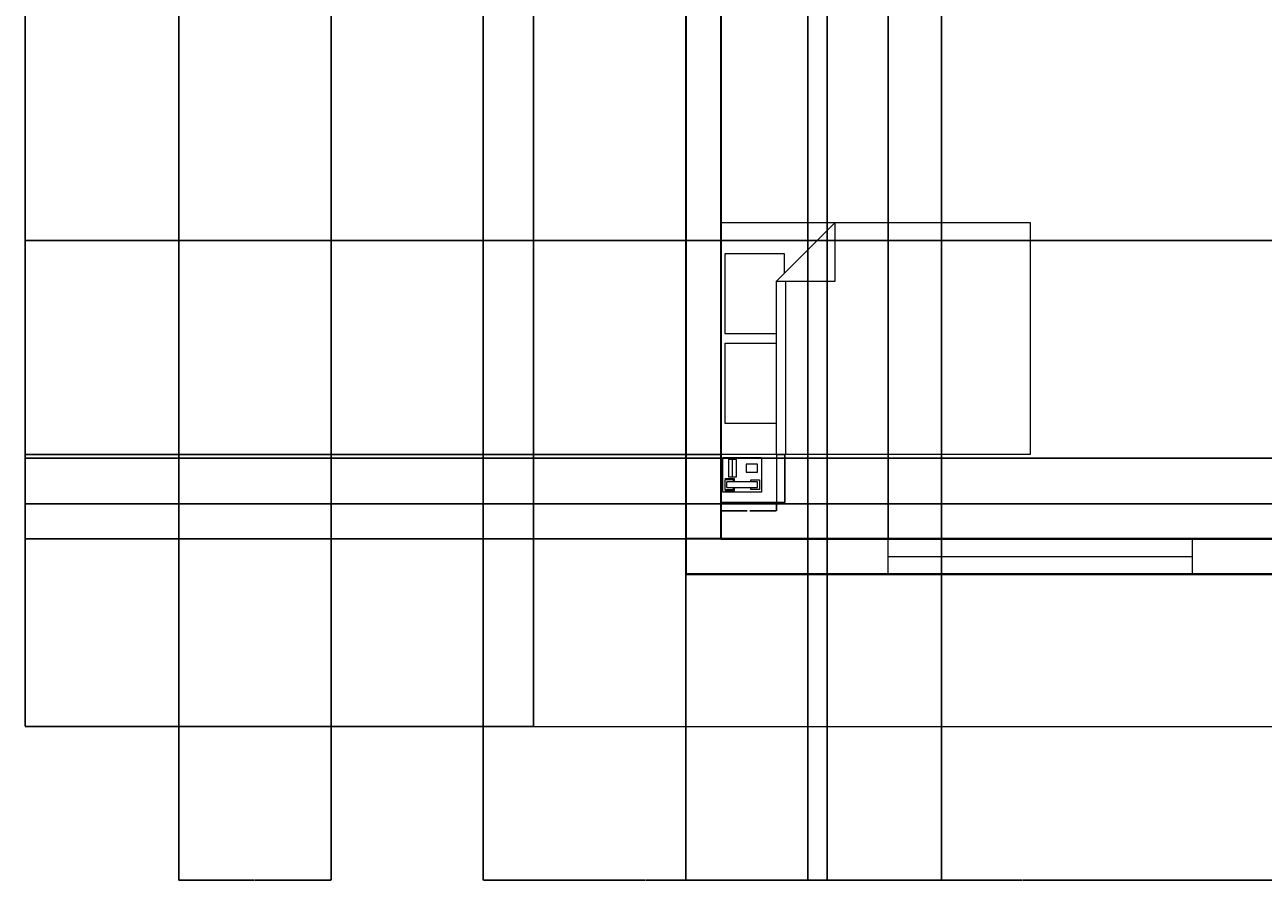
# Model space of a CAD drawing. Units: millimetres. Extents: x -8052 to 19968, y -37825 to -17505.
# Tile 1 of 10: x -8052 to 84, y -37825 to -32209. Entities that reach past the tile are written whole.
import ezdxf

# ---------------------------------------------------------------- set-up
doc = ezdxf.new("R2010")
doc.units = ezdxf.units.MM
doc.header["$MEASUREMENT"] = 0
for name, color, linetype, lineweight in [('A-ANNO-DIMS', 2, 'Continuous', 18), ('A-EQPM', 8, 'Continuous', 18), ('A-FLOR', 8, 'Continuous', 18), ('A-FURN', 8, 'Continuous', 18), ('A-GLAZ', 4, 'Continuous', 18), ('A-WALL', 7, 'Continuous', 35)]:
    doc.layers.add(name, color=color, linetype=linetype, lineweight=lineweight)
doc.styles.get("Standard").update_dxf_attribs({"font": 'arial.ttf'})
doc.dimstyles.get("Standard").update_dxf_attribs({"dimtxt": 1.054, "dimasz": 1.055, "dimexe": 0.18, "dimexo": 0.0625, "dimgap": 0.09, "dimtad": 0, "dimtih": 1, "dimtoh": 1, "dimdec": 4, "dimzin": 0, "dimdsep": 46, "dimtxsty": 'Standard', "dimcen": 0.09, "dimadec": 0, "dimazin": 0, "dimtfac": 1, "dimtdec": 4, "dimtofl": 0, "dimtmove": 0, "dimatfit": 3, "dimfxl": 1, "dimtolj": 1, "dimtzin": 0, "dimarcsym": 0})

# ---------------------------------------------------------------- blocks, each defined once
blk = doc.blocks.new('Bed - Queen')
for p, q in [((0, -80.00003), (0, 0)), ((0, 0), (59.99999, 0)), ((59.99999, 0), (59.99999, -80.00003)), ((7.99999, -1.2), (28.79998, -1.2)), ((7.99999, -14.4), (7.99999, -1.2)), ((28.79998, -1.2), (28.79998, -14.4)), ((31.19999, -1.2), (51.99999, -1.2)), ((31.19999, -14.4), (31.19999, -1.2)), ((51.99999, -1.2), (51.99999, -16.4)), ((0, -14.4), (44.8, -14.4)), ((59.99999, -29.6), (44.8, -14.4)), ((44.8, -14.4), (44.8, -29.6)), ((44.8, -16.8), (0, -16.8)), ((51.99999, -16.4), (46.79936, -16.4)), ((44.8, -29.6), (59.99999, -29.6)), ((59.99999, -80.00003), (0, -80.00003))]:
    blk.add_line(p, q)
blk = doc.blocks.new('Phone - Desk')
for p, q in [((-4.5, -5), (-4.5, 5)), ((-4.5, 5), (4.5, 5)), ((-4, 4.5), (-4, 2)), ((-3.75, 4.5), (-3.75, 2.25)), ((-1.25, 4.5), (-3.75, 4.5)), ((-3.25, 4), (-3.25, -4)), ((-3.25, 4), (-1.75, 4)), ((-1.75, -4), (-1.75, 4)), ((-1.25, 2.25), (-1.25, 4.5)), ((-1, 2), (-1, 4.5)), ((4, 3.5), (-0.5, 3.5)), ((-0.5, 3.5), (-0.5, 1.5)), ((4, 1.5), (4, 3.5)), ((4.5, 5), (4.5, -5)), ((-4, 2), (-3.25, 2)), ((-3.75, 2.25), (-3.25, 2.25)), ((-1.75, 2.25), (-1.25, 2.25)), ((-1.75, 2), (-1, 2)), ((-0.5, 2.5), (4, 2.5)), ((-0.5, 1.5), (4, 1.5)), ((-3.75, -2.25), (-3.25, -2.25)), ((-3.75, -4.5), (-3.75, -2.25)), ((-1.75, -2.25), (-1.25, -2.25)), ((-1.25, -2.25), (-1.25, -4.5)), ((2.75, -1), (0.75, -1)), ((0.75, -1), (0.75, -4)), ((2.75, -4), (2.75, -1)), ((4.5, -5), (-4.5, -5)), ((-1.25, -4.5), (-3.75, -4.5)), ((-3.25, -4), (-1.75, -4)), ((0.75, -4), (2.75, -4))]:
    blk.add_line(p, q)
blk = doc.blocks.new('TABLE-BEDSIDE')
for p, q in [((365.8, 315.3), (365.8, 0)), ((365.8, 0), (0, 0))]:
    blk.add_line(p, q)
blk = doc.blocks.new('WIN-2000')
for p, q in [((0, 0), (0, 230)), ((2000, 0), (2000, 230)), ((0, 115), (2000, 115))]:
    blk.add_line(p, q)
blk = doc.blocks.new('*D50')
at = {"layer": 'A-ANNO-DIMS', "color": 0, "lineweight": -2, "transparency": 16777216}
for p, q in [((-3480, -35345.8), (-3480, -35400.8)), ((-3114.3, -35345.8), (-3114.3, -35400.8)), ((-3479, -35400.6), (-3306.2, -35400.6)), ((-3115.3, -35400.6), (-3288.1, -35400.6))]:
    blk.add_line(p, q, dxfattribs=at)
at = {"layer": 'A-ANNO-DIMS', "color": 0, "lineweight": 100, "transparency": 16777216}
for points in [[(-3479, -35400.5), (-3479, -35400.8), (-3480, -35400.6)], [(-3115.3, -35400.5), (-3115.3, -35400.8), (-3114.3, -35400.6)]]:
    blk.add_solid(points, dxfattribs=at)
at = {"layer": 'Defpoints', "color": 0, "lineweight": 100, "transparency": 16777216}
for p in [(-3480, -35345.8), (-3114.3, -35345.8), (-3114.3, -35400.6)]:
    blk.add_point(p, dxfattribs=at)
at = {"layer": 'A-ANNO-DIMS', "color": 0, "transparency": 16777216, "insert": (-3297.1, -35400.6), "char_height": 1.054, "attachment_point": 5}
blk.add_mtext('\\A1;BEDSIDE TABLE 366 TYP.', dxfattribs=at)
blk = doc.blocks.new('*D51')
at = {"layer": 'A-ANNO-DIMS', "color": 0, "lineweight": -2, "transparency": 16777216}
for p, q in [((-3114.2, -35030.5), (-3059.2, -35030.5)), ((-3059.4, -35031.6), (-3059.4, -35187.5)), ((-3059.4, -35344.7), (-3059.4, -35188.8)), ((-3114.2, -35345.8), (-3059.2, -35345.8))]:
    blk.add_line(p, q, dxfattribs=at)
at = {"layer": 'A-ANNO-DIMS', "color": 0, "lineweight": 100, "transparency": 16777216}
for points in [[(-3059.6, -35031.6), (-3059.2, -35031.6), (-3059.4, -35030.5)], [(-3059.6, -35344.7), (-3059.2, -35344.7), (-3059.4, -35345.8)]]:
    blk.add_solid(points, dxfattribs=at)
at = {"layer": 'Defpoints', "color": 0, "lineweight": 100, "transparency": 16777216}
for p in [(-3114.3, -35030.5), (-3059.4, -35030.5), (-3114.3, -35345.8)]:
    blk.add_point(p, dxfattribs=at)
at = {"layer": 'A-ANNO-DIMS', "color": 0, "transparency": 16777216, "insert": (-3059.4, -35188.1), "char_height": 1.054, "attachment_point": 5}
blk.add_mtext('\\A1;315 TYP.', dxfattribs=at)
blk = doc.blocks.new('*D85')
at = {"layer": 'A-ANNO-DIMS', "color": 0, "lineweight": -2, "transparency": 16777216}
for p, q in [((-7040.1, -18514.8), (-8049.7, -18514.8)), ((-8049.5, -18515.9), (-8049.5, -27664.2)), ((-8049.5, -36813.8), (-8049.5, -27665.5)), ((-4710.1, -36814.8), (-8049.7, -36814.8))]:
    blk.add_line(p, q, dxfattribs=at)
at = {"layer": 'A-ANNO-DIMS', "color": 0, "lineweight": 100, "transparency": 16777216}
for points in [[(-8049.7, -18515.9), (-8049.3, -18515.9), (-8049.5, -18514.8)], [(-8049.7, -36813.8), (-8049.3, -36813.8), (-8049.5, -36814.8)]]:
    blk.add_solid(points, dxfattribs=at)
at = {"layer": 'Defpoints', "color": 0, "lineweight": 100, "transparency": 16777216}
for p in [(-7040, -18514.8), (-8049.5, -36814.8), (-4710, -36814.8)]:
    blk.add_point(p, dxfattribs=at)
at = {"layer": 'A-ANNO-DIMS', "color": 0, "transparency": 16777216, "insert": (-8049.5, -27664.8), "char_height": 1.05, "attachment_point": 5}
blk.add_mtext('\\A1;18300', dxfattribs=at)
blk = doc.blocks.new('*D86')
at = {"layer": 'A-ANNO-DIMS', "color": 0, "lineweight": -2, "transparency": 16777216}
for p, q in [((-7040, -18514.9), (-7040, -37824.5)), ((-6040, -19514.9), (-6040, -37824.5)), ((-7039, -37824.3), (-6541.6, -37824.3)), ((-6041.1, -37824.3), (-6538.4, -37824.3))]:
    blk.add_line(p, q, dxfattribs=at)
at = {"layer": 'A-ANNO-DIMS', "color": 0, "lineweight": 100, "transparency": 16777216}
for points in [[(-7039, -37824.2), (-7039, -37824.5), (-7040, -37824.3)], [(-6041.1, -37824.2), (-6041.1, -37824.5), (-6040, -37824.3)]]:
    blk.add_solid(points, dxfattribs=at)
at = {"layer": 'Defpoints', "color": 0, "lineweight": 100, "transparency": 16777216}
for p in [(-7040, -18514.8), (-6040, -19514.8), (-6040, -37824.3)]:
    blk.add_point(p, dxfattribs=at)
at = {"layer": 'A-ANNO-DIMS', "color": 0, "transparency": 16777216, "insert": (-6540, -37824.3), "char_height": 1.05, "attachment_point": 5}
blk.add_mtext('\\A1;1000', dxfattribs=at)
blk = doc.blocks.new('*D94')
at = {"layer": 'A-ANNO-DIMS', "color": 0, "lineweight": -2, "transparency": 16777216}
for p, q in [((-2780, -20744.9), (-2780, -37824.5)), ((-2030, -20744.9), (-2030, -37824.5)), ((-2779, -37824.3), (-2406.3, -37824.3)), ((-2031.1, -37824.3), (-2403.8, -37824.3))]:
    blk.add_line(p, q, dxfattribs=at)
at = {"layer": 'A-ANNO-DIMS', "color": 0, "lineweight": 100, "transparency": 16777216}
for points in [[(-2779, -37824.2), (-2779, -37824.5), (-2780, -37824.3)], [(-2031.1, -37824.2), (-2031.1, -37824.5), (-2030, -37824.3)]]:
    blk.add_solid(points, dxfattribs=at)
at = {"layer": 'Defpoints', "color": 0, "lineweight": 100, "transparency": 16777216}
for p in [(-2780, -20744.8), (-2030, -20744.8), (-2030, -37824.3)]:
    blk.add_point(p, dxfattribs=at)
at = {"layer": 'A-ANNO-DIMS', "color": 0, "transparency": 16777216, "insert": (-2405, -37824.3), "char_height": 1.05, "attachment_point": 5}
blk.add_mtext('\\A1;750', dxfattribs=at)
blk = doc.blocks.new('*D99')
at = {"layer": 'A-ANNO-DIMS', "color": 0, "lineweight": -2, "transparency": 16777216}
for p, q in [((-4710, -36814.8), (-4710, -17505.2)), ((-4709, -17505.3), (-4211.6, -17505.3)), ((-3711.1, -17505.3), (-4208.4, -17505.3)), ((-3710, -35814.8), (-3710, -17505.2))]:
    blk.add_line(p, q, dxfattribs=at)
at = {"layer": 'A-ANNO-DIMS', "color": 0, "lineweight": 100, "transparency": 16777216}
for points in [[(-4709, -17505.2), (-4709, -17505.5), (-4710, -17505.3)], [(-3711.1, -17505.2), (-3711.1, -17505.5), (-3710, -17505.3)]]:
    blk.add_solid(points, dxfattribs=at)
at = {"layer": 'Defpoints', "color": 0, "lineweight": 100, "transparency": 16777216}
for p in [(-3710, -17505.3), (-3710, -35814.8), (-4710, -36814.8)]:
    blk.add_point(p, dxfattribs=at)
at = {"layer": 'A-ANNO-DIMS', "color": 0, "transparency": 16777216, "insert": (-4210, -17505.3), "char_height": 1.05, "attachment_point": 5}
blk.add_mtext('\\A1;1000', dxfattribs=at)
blk = doc.blocks.new('*D100')
at = {"layer": 'A-ANNO-DIMS', "color": 0, "lineweight": -2, "transparency": 16777216}
for p, q in [((-3710, -35814.9), (-3710, -37824.5)), ((720, -35814.9), (720, -37824.5)), ((-3709, -37824.3), (-1496.7, -37824.3)), ((718.9, -37824.3), (-1493.3, -37824.3))]:
    blk.add_line(p, q, dxfattribs=at)
at = {"layer": 'A-ANNO-DIMS', "color": 0, "lineweight": 100, "transparency": 16777216}
for points in [[(-3709, -37824.2), (-3709, -37824.5), (-3710, -37824.3)], [(718.9, -37824.2), (718.9, -37824.5), (720, -37824.3)]]:
    blk.add_solid(points, dxfattribs=at)
at = {"layer": 'Defpoints', "color": 0, "lineweight": 100, "transparency": 16777216}
for p in [(-3710, -35814.8), (720, -35814.8), (720, -37824.3)]:
    blk.add_point(p, dxfattribs=at)
at = {"layer": 'A-ANNO-DIMS', "color": 0, "transparency": 16777216, "insert": (-1495, -37824.3), "char_height": 1.05, "attachment_point": 5}
blk.add_mtext('\\A1;4430', dxfattribs=at)
blk = doc.blocks.new('*D103')
at = {"layer": 'A-ANNO-DIMS', "color": 0, "lineweight": -2, "transparency": 16777216}
for p, q in [((-3480, -35584.8), (-3480, -17505.2)), ((-3479, -17505.3), (-2931.6, -17505.3)), ((-2381.1, -17505.3), (-2928.4, -17505.3)), ((-2380, -35584.8), (-2380, -17505.2))]:
    blk.add_line(p, q, dxfattribs=at)
at = {"layer": 'A-ANNO-DIMS', "color": 0, "lineweight": 100, "transparency": 16777216}
for points in [[(-3479, -17505.2), (-3479, -17505.5), (-3480, -17505.3)], [(-2381.1, -17505.2), (-2381.1, -17505.5), (-2380, -17505.3)]]:
    blk.add_solid(points, dxfattribs=at)
at = {"layer": 'Defpoints', "color": 0, "lineweight": 100, "transparency": 16777216}
for p in [(-2380, -17505.3), (-3480, -35584.8), (-2380, -35584.8)]:
    blk.add_point(p, dxfattribs=at)
at = {"layer": 'A-ANNO-DIMS', "color": 0, "transparency": 16777216, "insert": (-2930, -17505.3), "char_height": 1.05, "attachment_point": 5}
blk.add_mtext('\\A1;1100', dxfattribs=at)
blk = doc.blocks.new('*D117')
at = {"layer": 'A-ANNO-DIMS', "color": 0, "lineweight": -2, "transparency": 16777216}
for p, q in [((-3480.1, -35030.5), (-8049.7, -35030.5)), ((-8049.5, -35031.6), (-8049.5, -35307)), ((-8049.5, -35583.8), (-8049.5, -35308.3)), ((-3480.1, -35584.8), (-8049.7, -35584.8))]:
    blk.add_line(p, q, dxfattribs=at)
at = {"layer": 'A-ANNO-DIMS', "color": 0, "lineweight": 100, "transparency": 16777216}
for points in [[(-8049.7, -35031.6), (-8049.3, -35031.6), (-8049.5, -35030.5)], [(-8049.7, -35583.8), (-8049.3, -35583.8), (-8049.5, -35584.8)]]:
    blk.add_solid(points, dxfattribs=at)
at = {"layer": 'Defpoints', "color": 0, "lineweight": 100, "transparency": 16777216}
for p in [(-8049.5, -35030.5), (-3480, -35030.5), (-3480, -35584.8)]:
    blk.add_point(p, dxfattribs=at)
at = {"layer": 'A-ANNO-DIMS', "color": 0, "transparency": 16777216, "insert": (-8049.5, -35307.7), "char_height": 1.05, "attachment_point": 5}
blk.add_mtext('\\A1;554.3', dxfattribs=at)
blk = doc.blocks.new('*D119')
at = {"layer": 'A-ANNO-DIMS', "color": 0, "lineweight": -2, "transparency": 16777216}
for p, q in [((5749.9, -35054.8), (-8049.7, -35054.8)), ((-8049.5, -35055.9), (-8049.5, -35204.2)), ((-8049.5, -35353.8), (-8049.5, -35205.5)), ((5749.9, -35354.8), (-8049.7, -35354.8))]:
    blk.add_line(p, q, dxfattribs=at)
at = {"layer": 'A-ANNO-DIMS', "color": 0, "lineweight": 100, "transparency": 16777216}
for points in [[(-8049.7, -35055.9), (-8049.3, -35055.9), (-8049.5, -35054.8)], [(-8049.7, -35353.8), (-8049.3, -35353.8), (-8049.5, -35354.8)]]:
    blk.add_solid(points, dxfattribs=at)
at = {"layer": 'Defpoints', "color": 0, "lineweight": 100, "transparency": 16777216}
for p in [(5750, -35054.8), (-8049.5, -35354.8), (5750, -35354.8)]:
    blk.add_point(p, dxfattribs=at)
at = {"layer": 'A-ANNO-DIMS', "color": 0, "transparency": 16777216, "insert": (-8049.5, -35204.8), "char_height": 1.05, "attachment_point": 5}
blk.add_mtext('\\A1;300', dxfattribs=at)
blk = doc.blocks.new('*D120')
at = {"layer": 'A-ANNO-DIMS', "color": 0, "lineweight": -2, "transparency": 16777216}
for p, q in [((949.9, -33624.8), (-8049.7, -33624.8)), ((-8049.5, -33625.9), (-8049.5, -34339.2)), ((-8049.5, -35053.8), (-8049.5, -34340.5)), ((949.9, -35054.8), (-8049.7, -35054.8))]:
    blk.add_line(p, q, dxfattribs=at)
at = {"layer": 'A-ANNO-DIMS', "color": 0, "lineweight": 100, "transparency": 16777216}
for points in [[(-8049.7, -33625.9), (-8049.3, -33625.9), (-8049.5, -33624.8)], [(-8049.7, -35053.8), (-8049.3, -35053.8), (-8049.5, -35054.8)]]:
    blk.add_solid(points, dxfattribs=at)
at = {"layer": 'Defpoints', "color": 0, "lineweight": 100, "transparency": 16777216}
for p in [(950, -33624.8), (-8049.5, -35054.8), (950, -35054.8)]:
    blk.add_point(p, dxfattribs=at)
at = {"layer": 'A-ANNO-DIMS', "color": 0, "transparency": 16777216, "insert": (-8049.5, -34339.8), "char_height": 1.05, "attachment_point": 5}
blk.add_mtext('\\A1;1430', dxfattribs=at)
blk = doc.blocks.new('*D125')
at = {"layer": 'A-ANNO-DIMS', "color": 0, "lineweight": -2, "transparency": 16777216}
for p, q in [((-5040, -25474.9), (-5040, -37824.5)), ((-2907.5, -25474.9), (-2907.5, -37824.5)), ((-5039, -37824.3), (-3976.1, -37824.3)), ((-2908.6, -37824.3), (-3971.5, -37824.3))]:
    blk.add_line(p, q, dxfattribs=at)
at = {"layer": 'A-ANNO-DIMS', "color": 0, "lineweight": 100, "transparency": 16777216}
for points in [[(-5039, -37824.2), (-5039, -37824.5), (-5040, -37824.3)], [(-2908.6, -37824.2), (-2908.6, -37824.5), (-2907.5, -37824.3)]]:
    blk.add_solid(points, dxfattribs=at)
at = {"layer": 'Defpoints', "color": 0, "lineweight": 100, "transparency": 16777216}
for p in [(-5040, -25474.8), (-2907.5, -25474.8), (-2907.5, -37824.3)]:
    blk.add_point(p, dxfattribs=at)
at = {"layer": 'A-ANNO-DIMS', "color": 0, "transparency": 16777216, "insert": (-3973.8, -37824.3), "char_height": 1.05, "attachment_point": 5}
blk.add_mtext('\\A1;2132.5', dxfattribs=at)

msp = doc.modelspace()

# ---------------------------------------------------------------- linework, layer by layer
at = {"layer": 'A-FLOR'}
for p, q in [((-4710.021, -26474.843), (-4710.021, -36814.843)), ((-4710.021, -36814.843), (11409.979, -36814.843))]:
    msp.add_line(p, q, dxfattribs=at)
at = {"layer": 'A-WALL'}
for p, q in [((-3710.021, -29974.843), (-3710.021, -35814.843)), ((-3480.021, -30204.843), (-3480.021, -35584.843)), ((10179.979, -35584.843), (-3710.021, -35584.843)), ((-3480.021, -35584.843), (10409.979, -35584.843)), ((-3710.021, -35814.843), (10409.979, -35814.843)), ((10409.979, -35814.843), (-3710.021, -35814.843))]:
    msp.add_line(p, q, dxfattribs=at)

# ---------------------------------------------------------------- block references
at = {"layer": 'A-EQPM', "xscale": 25.4, "yscale": 25.4, "zscale": 25.4, "rotation": 90}
msp.add_blockref('Phone - Desk', (-3338.76, -35164.132), dxfattribs=at)
at = {"layer": 'A-FURN', "xscale": 25.4, "yscale": 25.4, "zscale": 25.4, "rotation": 90}
msp.add_blockref('Bed - Queen', (-3480.021, -35030.504), dxfattribs=at)
at = {"layer": 'A-FURN'}
msp.add_blockref('TABLE-BEDSIDE', (-3480.021, -35345.763), dxfattribs=at)
at = {"layer": 'A-GLAZ'}
msp.add_blockref('WIN-2000', (-2380.021, -35814.843), dxfattribs=at)

# ---------------------------------------------------------------- dimensions: what is measured, and where the dimension line sits
at = {"layer": 'A-ANNO-DIMS'}
for base, p1, p2, override, picture, middle in [((-3710.021, -17505.343), (-4710.021, -36814.843), (-3710.021, -35814.843), {"dimdec": 0, "dimlfac": 1, "dimrnd": 0, "dimzin": 0, "dimdsep": 46, "dimlunit": 2}, '*D99', (-4210.021, -17505.343)), ((-2380.021, -17505.343), (-3480.021, -35584.843), (-2380.021, -35584.843), {"dimdec": 0, "dimlfac": 1, "dimrnd": 0, "dimzin": 0, "dimdsep": 46, "dimlunit": 2}, '*D103', (-2930.021, -17505.343)), ((-6040.021, -37824.343), (-7040.021, -18514.843), (-6040.021, -19514.843), {"dimdec": 0, "dimlfac": 1, "dimrnd": 0, "dimzin": 0, "dimdsep": 46, "dimlunit": 2}, '*D86', (-6540.021, -37824.343)), ((-2030.021, -37824.343), (-2780.021, -20744.843), (-2030.021, -20744.843), {"dimdec": 0, "dimlfac": 1, "dimrnd": 0, "dimzin": 0, "dimdsep": 46, "dimlunit": 2}, '*D94', (-2405.021, -37824.343)), ((-2907.521, -37824.343), (-5040.021, -25474.843), (-2907.521, -25474.843), {"dimdec": 1, "dimlfac": 1, "dimrnd": 0, "dimzin": 0, "dimdsep": 46, "dimlunit": 2}, '*D125', (-3973.771, -37824.343)), ((719.979, -37824.343), (-3710.021, -35814.843), (719.979, -35814.843), {"dimdec": 0, "dimlfac": 1, "dimrnd": 0, "dimzin": 0, "dimdsep": 46, "dimlunit": 2}, '*D100', (-1495.021, -37824.343))]:
    dim = msp.add_linear_dim(base=base, p1=p1, p2=p2, dimstyle='Standard', override=override, dxfattribs=at)
    dim.commit()
    dim.dimension.update_dxf_attribs({"geometry": picture, "text_midpoint": middle})
for base, p1, p2, override, picture, middle in [((-8049.521, -36814.843), (-7040.021, -18514.843), (-4710.021, -36814.843), {"dimdec": 0, "dimlfac": 1, "dimrnd": 0, "dimzin": 0, "dimdsep": 46, "dimlunit": 2}, '*D85', (-8049.521, -27664.843)), ((-8049.521, -35054.843), (949.979, -33624.843), (949.979, -35054.843), {"dimdec": 0, "dimlfac": 1, "dimrnd": 0, "dimzin": 0, "dimdsep": 46, "dimlunit": 2}, '*D120', (-8049.521, -34339.843)), ((-8049.521, -35030.504), (-3480.021, -35584.843), (-3480.021, -35030.504), {"dimdec": 1, "dimlfac": 1, "dimrnd": 0, "dimzin": 0, "dimdsep": 46, "dimlunit": 2}, '*D117', (-8049.521, -35307.674)), ((-8049.521, -35354.843), (5749.979, -35054.843), (5749.979, -35354.843), {"dimdec": 0, "dimlfac": 1, "dimrnd": 0, "dimzin": 0, "dimdsep": 46, "dimlunit": 2}, '*D119', (-8049.521, -35204.843))]:
    dim = msp.add_linear_dim(base=base, p1=p1, p2=p2, angle=90, dimstyle='Standard', override=override, dxfattribs=at)
    dim.commit()
    dim.dimension.update_dxf_attribs({"geometry": picture, "text_midpoint": middle})
dim = msp.add_linear_dim(base=(-3059.397, -35030.504), p1=(-3114.261, -35345.763), p2=(-3114.261, -35030.504), angle=90, text='<> TYP.', dimstyle='Standard', override={"dimdec": 0, "dimlfac": 1, "dimrnd": 0, "dimzin": 0, "dimdsep": 46, "dimlunit": 2}, dxfattribs=at)
dim.commit()
dim.dimension.update_dxf_attribs({"geometry": '*D51', "text_midpoint": (-3059.397, -35188.134)})
dim = msp.add_linear_dim(base=(-3114.261, -35400.627), p1=(-3480.021, -35345.763), p2=(-3114.261, -35345.763), text='BEDSIDE TABLE <> TYP.', dimstyle='Standard', override={"dimdec": 0, "dimlfac": 1, "dimrnd": 0, "dimzin": 0, "dimdsep": 46, "dimlunit": 2}, dxfattribs=at)
dim.commit()
dim.dimension.update_dxf_attribs({"geometry": '*D50', "text_midpoint": (-3297.141, -35400.627)})

doc.saveas('drawing.dxf')
